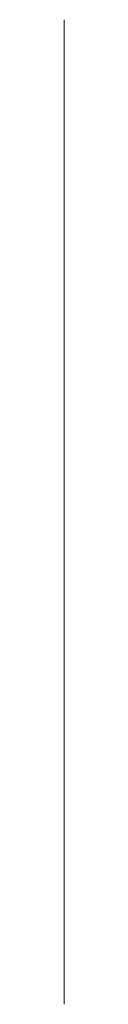
# Model space of a CAD drawing. Units: millimetres. Extents: x 0 to 3678, y 1592 to 1922.
# Tile 1 of 2: x 0 to 0, y 1666 to 1716. Entities that reach past the tile are written whole.
import ezdxf

# ---------------------------------------------------------------- set-up
doc = ezdxf.new("R2010")
doc.units = ezdxf.units.MM
doc.layers.add('M-CONS', color=8, linetype='Continuous', lineweight=18)

msp = doc.modelspace()

# ---------------------------------------------------------------- linework, layer by layer
at = {"layer": 'M-CONS', "extrusion": (1, 0, 0)}
for p, q in [((0, 1716.125, 6.099), (0, 1716.125, -83.901)), ((0, 1716.125, -83.901), (0, 1666.125, -83.901)), ((0, 1716.125, -83.901), (0, 1716.125, -63.901)), ((0, 1716.125, 6.099), (0, 1716.125, 26.099)), ((0, 1716.125, 26.099), (0, 1666.125, 26.099)), ((0, 1666.125, -83.901), (0, 1666.125, 6.099)), ((0, 1666.125, 26.099), (0, 1666.125, 6.099))]:
    msp.add_line(p, q, dxfattribs=at)
for centre in [(1696.125, 6.099), (1696.125, -63.901)]:
    msp.add_circle(centre, 8, dxfattribs=at)

doc.saveas('drawing.dxf')
